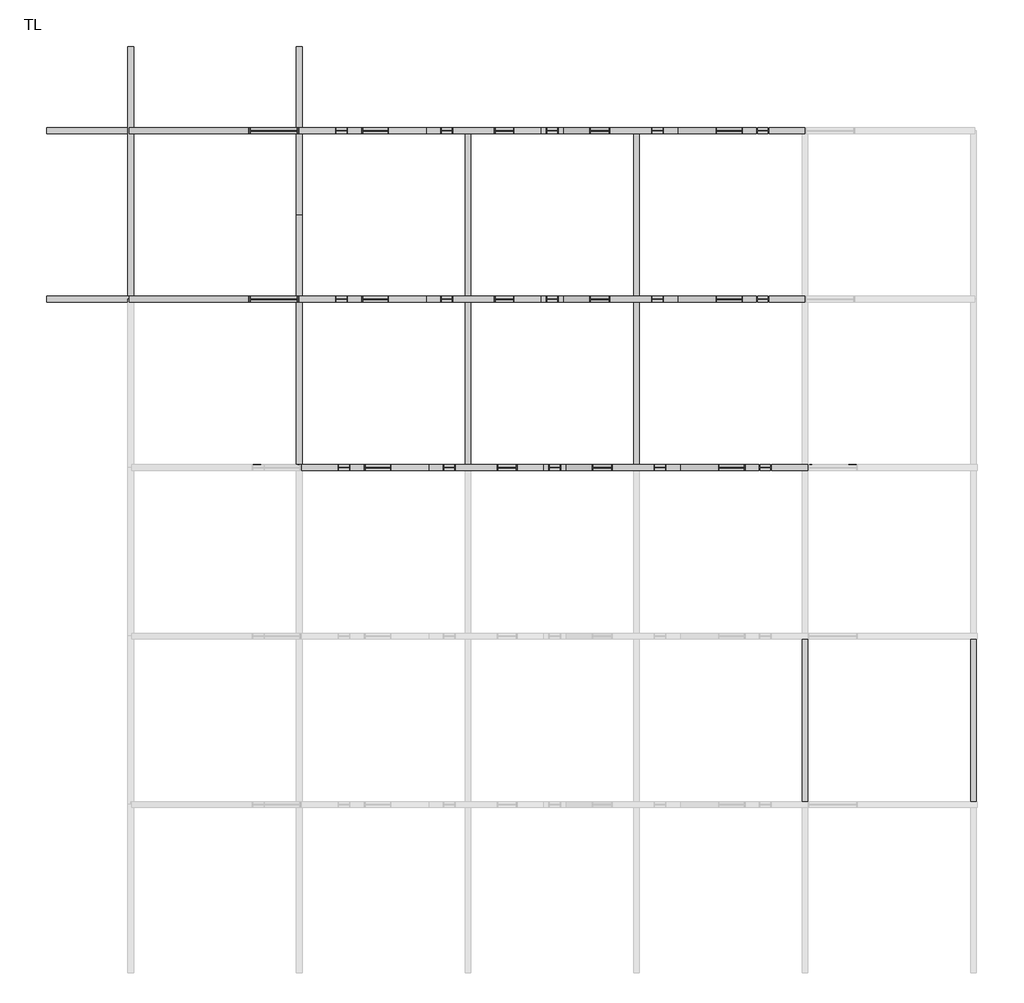
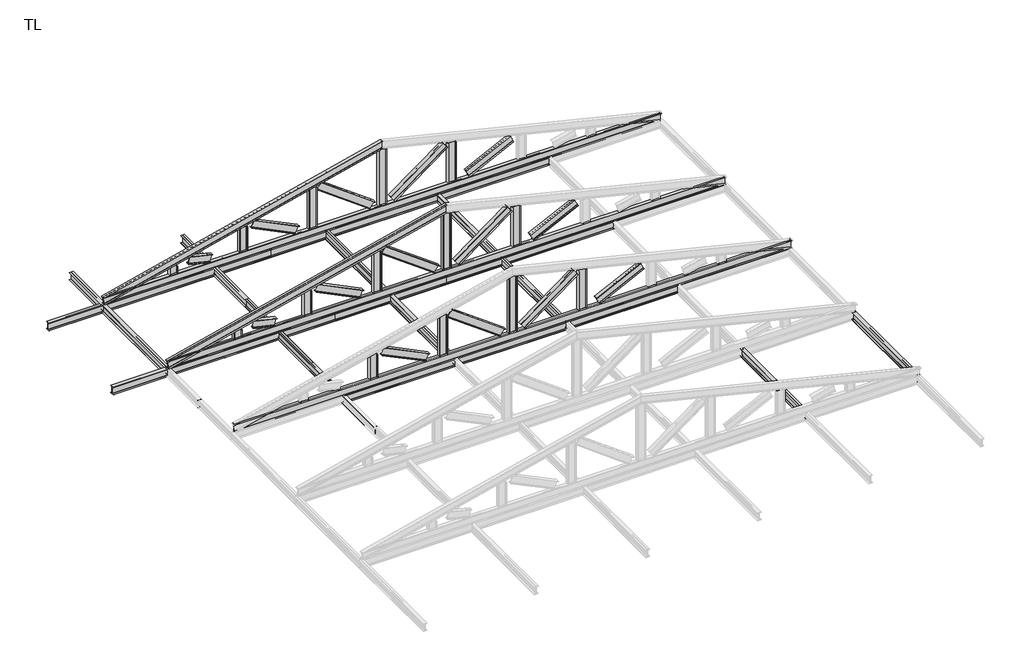
# One storey, part 3 of 4: 53 beams.
"""IFC4 building model written with IfcOpenShell, lengths in millimetres."""

from ifc_helpers import new_model, si_unit, frame, origin, place, context, project, spatial, polyline, circle_curve, ellipse_curve, transform, mapped, element, save
from ifc_brep_helpers import plane_surface, revolved_surface, advanced_brep
from components import w_shapes_w14x30_541e514d, w_shapes_w14x30_920474df, w_shapes_w14x30_f0ef5163, w_shapes_w14x30_e8a2e8cf, w_shapes_w14x30_72b19b1b, w_shapes_w14x30_b44ec7f2, w_shapes_w14x30_809da129, w_shapes_w14x30_b6c746c8, w_shapes_w14x30_333ad3b1, w_shapes_w14x30_a113fbeb, w_shapes_w14x30_23e28ad8, w_shapes_w14x30_8f152a7c

model = new_model("IFC4")

# Units and contexts
model_context = context("Model", 3, world=origin())
ifc_project = project(units=[si_unit("LENGTHUNIT", "METRE", prefix="MILLI")], contexts=[model_context])

# Site, building, storey
site = spatial("IfcSite", under=ifc_project)
building = spatial("IfcBuilding", under=site)
storey = spatial("IfcBuildingStorey", under=building, Name="TL", Elevation=8534.4)

# Beams
placement = place(None, origin())
element("IfcBeam", 1, ObjectType="W Shapes : W14X30", at=placement, inside=storey, context=model_context, shape_type="AdvancedBrep", body=[
    advanced_brep(
    [(-18386.4356148, 14124.3335479, 8538.7295322), (-18384.1189802, 14124.3335479, 8529.2288983), (-18384.1189802, 13953.3915479, 8529.2288983), (-18386.4356148, 13953.3915479, 8538.7295322), (-18386.4356148, 14025.2735479, 8538.7295322), (-18388.8425079, 14035.4335479, 8548.6003207), (-18462.4332635, 14035.4335479, 8850.3996793), (-18464.8401565, 14025.2735479, 8860.2704678), (-18464.8401565, 13953.3915479, 8860.2704678), (-18467.1567911, 13953.3915479, 8869.7711017), (-18467.1567911, 14124.3335479, 8869.7711017), (-18464.8401565, 14124.3335479, 8860.2704678), (-18464.8401565, 14052.4515479, 8860.2704678), (-18462.4332635, 14042.2915479, 8850.3996793), (-18388.8425079, 14042.2915479, 8548.6003207), (-18386.4356148, 14052.4515479, 8538.7295322), (-5925.6378857, 14052.4515479, 11577.1704505), (-5925.6378857, 14124.3335479, 11577.1704505), (-5925.6378857, 14042.2915479, 11587.6281358), (-5925.6378857, 14042.2915479, 11907.3718642), (-5925.6378857, 14052.4515479, 11917.8295495), (-5925.6378857, 14124.3335479, 11917.8295495), (-5925.6378857, 14124.3335479, 11927.8950717), (-5925.6378857, 13953.3915479, 11927.8950717), (-5925.6378857, 13953.3915479, 11917.8295495), (-5925.6378857, 14025.2735479, 11917.8295495), (-5925.6378857, 14035.4335479, 11907.3718642), (-5925.6378857, 14035.4335479, 11587.6281358), (-5925.6378857, 14025.2735479, 11577.1704505), (-5925.6378857, 13953.3915479, 11577.1704505), (-5925.6378857, 13953.3915479, 11567.1049283), (-5925.6378857, 14124.3335479, 11567.1049283)],
    [
        (0, 1),
        (1, 2),
        (2, 3),
        (3, 4),
        (4, 5, circle_curve(frame((-18388.8425079, 14025.2735479, 8548.6003207), z_axis=(0.971534301878756, 0.0, 0.23689892417011604), x_axis=(0.23689892417011604, 0.0, -0.971534301878756)), 10.16)),
        (5, 6),
        (6, 7, circle_curve(frame((-18462.4332635, 14025.2735479, 8850.3996793), z_axis=(0.971534301878756, 0.0, 0.23689892417011604), x_axis=(0.0, 1.0000000000000002, 0.0)), 10.16)),
        (7, 8),
        (8, 9),
        (9, 10),
        (10, 11),
        (11, 12),
        (12, 13, circle_curve(frame((-18462.4332635, 14052.4515479, 8850.3996793), z_axis=(0.971534301878756, 0.0, 0.23689892417011604), x_axis=(-0.23689892417011604, 0.0, 0.971534301878756)), 10.16)),
        (13, 14),
        (14, 15, circle_curve(frame((-18388.8425079, 14052.4515479, 8548.6003207), z_axis=(0.971534301878756, 0.0, 0.23689892417011604), x_axis=(0.0, -1.0000000000000002, 0.0)), 10.16)),
        (15, 0),
        (16, 17),
        (17, 0),
        (15, 16),
        (18, 16, ellipse_curve(frame((-5925.6378857, 14052.4515479, 11587.6281358), z_axis=(1.0, 0.0, 0.0), x_axis=(0.0, 0.0, -1.0)), 10.4576853, 10.16)),
        (14, 18),
        (19, 18),
        (13, 19),
        (20, 19, ellipse_curve(frame((-5925.6378857, 14052.4515479, 11907.3718642), z_axis=(1.0, 0.0, 0.0), x_axis=(0.0, 0.0, -1.0)), 10.4576853, 10.16)),
        (12, 20),
        (21, 20),
        (11, 21),
        (22, 21),
        (10, 22),
        (23, 22),
        (9, 23),
        (24, 23),
        (8, 24),
        (25, 24),
        (7, 25),
        (26, 25, ellipse_curve(frame((-5925.6378857, 14025.2735479, 11907.3718642), z_axis=(1.0, 0.0, 0.0), x_axis=(0.0, 0.0, -1.0)), 10.4576853, 10.16)),
        (6, 26),
        (27, 26),
        (5, 27),
        (28, 27, ellipse_curve(frame((-5925.6378857, 14025.2735479, 11587.6281358), z_axis=(1.0, 0.0, 0.0), x_axis=(0.0, 0.0, -1.0)), 10.4576853, 10.16)),
        (4, 28),
        (29, 28),
        (3, 29),
        (30, 29),
        (2, 30),
        (31, 30),
        (1, 31),
        (17, 31),
    ],
    [
        plane_surface(frame((-18425.6378857, 14038.8625479, 8699.5), z_axis=(-0.971534301878756, 0.0, -0.23689892417011604), x_axis=(-0.23689892417011604, 0.0, 0.971534301878756))),
        plane_surface(frame((-5886.4356148, 14088.3925479, 11586.7295322), z_axis=(-0.23689892417011604, 0.0, 0.971534301878756), x_axis=(0.0, -1.0, 0.0))),
        revolved_surface(polyline([(-18388.8425079, 14042.2915479, 8548.600320699998), (-5923.230992628227, 14042.2915479, 11588.215032583868)]), (-5888.8425079, 14052.4515479, 11596.6003207), (-0.971534301878756, 0.0, -0.23689892417011604)),
        plane_surface(frame((-5925.6378857, 14042.2915479, 11747.5), z_axis=(0.0, 1.0000000000000002, 0.0), x_axis=(-0.23689892417011604, 0.0, 0.971534301878756))),
        revolved_surface(polyline([(-18464.840156569568, 14052.4515479, 8860.270467807088), (-5925.637885708268, 14052.4515479, 11917.82954953391)]), (-5962.4332635, 14052.4515479, 11898.3996793), (-0.971534301878756, 0.0, -0.23689892417011604)),
        plane_surface(frame((-5964.8401565, 14088.3925479, 11908.2704678), z_axis=(0.23689892417011604, 0.0, -0.971534301878756), x_axis=(0.0, 1.0, 0.0))),
        plane_surface(frame((-5965.9984738, 14124.3335479, 11913.0207848), z_axis=(0.0, 1.0000000000000002, 0.0), x_axis=(-0.23689892417011604, 0.0, 0.971534301878756))),
        plane_surface(frame((-5967.1567911, 14038.8625479, 11917.7711017), z_axis=(-0.23689892417011604, 0.0, 0.971534301878756), x_axis=(0.0, -1.0, 0.0))),
        plane_surface(frame((-5965.9984738, 13953.3915479, 11913.0207848), z_axis=(0.0, -1.0000000000000002, 0.0), x_axis=(0.23689892417011604, 0.0, -0.971534301878756))),
        plane_surface(frame((-5964.8401565, 13989.3325479, 11908.2704678), z_axis=(0.23689892417011604, 0.0, -0.971534301878756), x_axis=(0.0, 1.0, 0.0))),
        revolved_surface(polyline([(-18462.4332635, 14035.4335479, 8850.399679299999), (-5923.2309926387, 14035.4335479, 11907.95876102682)]), (-5962.4332635, 14025.2735479, 11898.3996793), (-0.971534301878756, 0.0, -0.23689892417011604)),
        plane_surface(frame((-5925.6378857, 14035.4335479, 11747.5), z_axis=(0.0, -1.0000000000000002, 0.0), x_axis=(0.23689892417011604, 0.0, -0.971534301878756))),
        revolved_surface(polyline([(-18386.435614830432, 14025.2735479, 8538.729532192909), (-5920.824099558658, 14025.2735479, 11578.34424407678)]), (-5888.8425079, 14025.2735479, 11596.6003207), (-0.971534301878756, 0.0, -0.23689892417011604)),
        plane_surface(frame((-5886.4356148, 13989.3325479, 11586.7295322), z_axis=(-0.23689892417011604, 0.0, 0.971534301878756), x_axis=(0.0, -1.0, 0.0))),
        plane_surface(frame((-5885.2772975, 13953.3915479, 11581.9792152), z_axis=(0.0, -1.0000000000000002, 0.0), x_axis=(0.23689892417011604, 0.0, -0.971534301878756))),
        plane_surface(frame((-5884.1189802, 14038.8625479, 11577.2288983), z_axis=(0.23689892417011604, 0.0, -0.971534301878756), x_axis=(0.0, 1.0, 0.0))),
        plane_surface(frame((-5885.2772975, 14124.3335479, 11581.9792152), z_axis=(0.0, 1.0000000000000002, 0.0), x_axis=(-0.23689892417011604, 0.0, 0.971534301878756))),
        plane_surface(frame((-5925.6378857, 14038.8625479, 11927.8950717), z_axis=(1.0, 0.0, 0.0), x_axis=(0.0, -1.0, 0.0))),
    ],
    [
        (0, [[1, 2, 3, 4, 5, 6, 7, 8, 9, 10, 11, 12, 13, 14, 15, 16]]),
        (1, [[17, 18, -16, 19]]),
        (2, [[20, -19, -15, 21]]),
        (3, [[22, -21, -14, 23]]),
        (4, [[24, -23, -13, 25]]),
        (5, [[26, -25, -12, 27]]),
        (6, [[28, -27, -11, 29]]),
        (7, [[30, -29, -10, 31]]),
        (8, [[32, -31, -9, 33]]),
        (9, [[34, -33, -8, 35]]),
        (10, [[36, -35, -7, 37]]),
        (11, [[38, -37, -6, 39]]),
        (12, [[40, -39, -5, 41]]),
        (13, [[42, -41, -4, 43]]),
        (14, [[44, -43, -3, 45]]),
        (15, [[46, -45, -2, 47]]),
        (16, [[48, -47, -1, -18]]),
        (17, [[-17, -20, -22, -24, -26, -28, -30, -32, -34, -36, -38, -40, -42, -44, -46, -48]]),
    ],
),
])
element("IfcBeam", 2, ObjectType="W Shapes : W14X30", at=placement, inside=storey, context=model_context, shape_type="AdvancedBrep", body=[
    advanced_brep(
    [(-18386.4356148, 19124.3335479, 8538.7295322), (-18384.1189802, 19124.3335479, 8529.2288983), (-18384.1189802, 18953.3915479, 8529.2288983), (-18386.4356148, 18953.3915479, 8538.7295322), (-18386.4356148, 19025.2735479, 8538.7295322), (-18388.8425079, 19035.4335479, 8548.6003207), (-18462.4332635, 19035.4335479, 8850.3996793), (-18464.8401565, 19025.2735479, 8860.2704678), (-18464.8401565, 18953.3915479, 8860.2704678), (-18467.1567911, 18953.3915479, 8869.7711017), (-18467.1567911, 19124.3335479, 8869.7711017), (-18464.8401565, 19124.3335479, 8860.2704678), (-18464.8401565, 19052.4515479, 8860.2704678), (-18462.4332635, 19042.2915479, 8850.3996793), (-18388.8425079, 19042.2915479, 8548.6003207), (-18386.4356148, 19052.4515479, 8538.7295322), (-5925.6378857, 19052.4515479, 11577.1704505), (-5925.6378857, 19124.3335479, 11577.1704505), (-5925.6378857, 19042.2915479, 11587.6281358), (-5925.6378857, 19042.2915479, 11907.3718642), (-5925.6378857, 19052.4515479, 11917.8295495), (-5925.6378857, 19124.3335479, 11917.8295495), (-5925.6378857, 19124.3335479, 11927.8950717), (-5925.6378857, 18953.3915479, 11927.8950717), (-5925.6378857, 18953.3915479, 11917.8295495), (-5925.6378857, 19025.2735479, 11917.8295495), (-5925.6378857, 19035.4335479, 11907.3718642), (-5925.6378857, 19035.4335479, 11587.6281358), (-5925.6378857, 19025.2735479, 11577.1704505), (-5925.6378857, 18953.3915479, 11577.1704505), (-5925.6378857, 18953.3915479, 11567.1049283), (-5925.6378857, 19124.3335479, 11567.1049283)],
    [
        (0, 1),
        (1, 2),
        (2, 3),
        (3, 4),
        (4, 5, circle_curve(frame((-18388.8425079, 19025.2735479, 8548.6003207), z_axis=(0.971534301878756, 0.0, 0.23689892417011604), x_axis=(0.23689892417011604, 0.0, -0.971534301878756)), 10.16)),
        (5, 6),
        (6, 7, circle_curve(frame((-18462.4332635, 19025.2735479, 8850.3996793), z_axis=(0.971534301878756, 0.0, 0.23689892417011604), x_axis=(0.0, 1.0000000000000002, 0.0)), 10.16)),
        (7, 8),
        (8, 9),
        (9, 10),
        (10, 11),
        (11, 12),
        (12, 13, circle_curve(frame((-18462.4332635, 19052.4515479, 8850.3996793), z_axis=(0.971534301878756, 0.0, 0.23689892417011604), x_axis=(-0.23689892417011604, 0.0, 0.971534301878756)), 10.16)),
        (13, 14),
        (14, 15, circle_curve(frame((-18388.8425079, 19052.4515479, 8548.6003207), z_axis=(0.971534301878756, 0.0, 0.23689892417011604), x_axis=(0.0, -1.0000000000000002, 0.0)), 10.16)),
        (15, 0),
        (16, 17),
        (17, 0),
        (15, 16),
        (18, 16, ellipse_curve(frame((-5925.6378857, 19052.4515479, 11587.6281358), z_axis=(1.0, 0.0, 0.0), x_axis=(0.0, 0.0, -1.0)), 10.4576853, 10.16)),
        (14, 18),
        (19, 18),
        (13, 19),
        (20, 19, ellipse_curve(frame((-5925.6378857, 19052.4515479, 11907.3718642), z_axis=(1.0, 0.0, 0.0), x_axis=(0.0, 0.0, -1.0)), 10.4576853, 10.16)),
        (12, 20),
        (21, 20),
        (11, 21),
        (22, 21),
        (10, 22),
        (23, 22),
        (9, 23),
        (24, 23),
        (8, 24),
        (25, 24),
        (7, 25),
        (26, 25, ellipse_curve(frame((-5925.6378857, 19025.2735479, 11907.3718642), z_axis=(1.0, 0.0, 0.0), x_axis=(0.0, 0.0, -1.0)), 10.4576853, 10.16)),
        (6, 26),
        (27, 26),
        (5, 27),
        (28, 27, ellipse_curve(frame((-5925.6378857, 19025.2735479, 11587.6281358), z_axis=(1.0, 0.0, 0.0), x_axis=(0.0, 0.0, -1.0)), 10.4576853, 10.16)),
        (4, 28),
        (29, 28),
        (3, 29),
        (30, 29),
        (2, 30),
        (31, 30),
        (1, 31),
        (17, 31),
    ],
    [
        plane_surface(frame((-18425.6378857, 19038.8625479, 8699.5), z_axis=(-0.971534301878756, 0.0, -0.23689892417011604), x_axis=(-0.23689892417011604, 0.0, 0.971534301878756))),
        plane_surface(frame((-5886.4356148, 19088.3925479, 11586.7295322), z_axis=(-0.23689892417011604, 0.0, 0.971534301878756), x_axis=(0.0, -1.0, 0.0))),
        revolved_surface(polyline([(-18388.8425079, 19042.2915479, 8548.600320699998), (-5923.230992628227, 19042.2915479, 11588.215032583868)]), (-5888.8425079, 19052.4515479, 11596.6003207), (-0.971534301878756, 0.0, -0.23689892417011604)),
        plane_surface(frame((-5925.6378857, 19042.2915479, 11747.5), z_axis=(0.0, 1.0000000000000002, 0.0), x_axis=(-0.23689892417011604, 0.0, 0.971534301878756))),
        revolved_surface(polyline([(-18464.840156569568, 19052.4515479, 8860.270467807088), (-5925.637885708268, 19052.4515479, 11917.82954953391)]), (-5962.4332635, 19052.4515479, 11898.3996793), (-0.971534301878756, 0.0, -0.23689892417011604)),
        plane_surface(frame((-5964.8401565, 19088.3925479, 11908.2704678), z_axis=(0.23689892417011604, 0.0, -0.971534301878756), x_axis=(0.0, 1.0, 0.0))),
        plane_surface(frame((-5965.9984738, 19124.3335479, 11913.0207848), z_axis=(0.0, 1.0000000000000002, 0.0), x_axis=(-0.23689892417011604, 0.0, 0.971534301878756))),
        plane_surface(frame((-5967.1567911, 19038.8625479, 11917.7711017), z_axis=(-0.23689892417011604, 0.0, 0.971534301878756), x_axis=(0.0, -1.0, 0.0))),
        plane_surface(frame((-5965.9984738, 18953.3915479, 11913.0207848), z_axis=(0.0, -1.0000000000000002, 0.0), x_axis=(0.23689892417011604, 0.0, -0.971534301878756))),
        plane_surface(frame((-5964.8401565, 18989.3325479, 11908.2704678), z_axis=(0.23689892417011604, 0.0, -0.971534301878756), x_axis=(0.0, 1.0, 0.0))),
        revolved_surface(polyline([(-18462.4332635, 19035.4335479, 8850.399679299999), (-5923.2309926387, 19035.4335479, 11907.95876102682)]), (-5962.4332635, 19025.2735479, 11898.3996793), (-0.971534301878756, 0.0, -0.23689892417011604)),
        plane_surface(frame((-5925.6378857, 19035.4335479, 11747.5), z_axis=(0.0, -1.0000000000000002, 0.0), x_axis=(0.23689892417011604, 0.0, -0.971534301878756))),
        revolved_surface(polyline([(-18386.435614830432, 19025.2735479, 8538.729532192909), (-5920.824099558658, 19025.2735479, 11578.34424407678)]), (-5888.8425079, 19025.2735479, 11596.6003207), (-0.971534301878756, 0.0, -0.23689892417011604)),
        plane_surface(frame((-5886.4356148, 18989.3325479, 11586.7295322), z_axis=(-0.23689892417011604, 0.0, 0.971534301878756), x_axis=(0.0, -1.0, 0.0))),
        plane_surface(frame((-5885.2772975, 18953.3915479, 11581.9792152), z_axis=(0.0, -1.0000000000000002, 0.0), x_axis=(0.23689892417011604, 0.0, -0.971534301878756))),
        plane_surface(frame((-5884.1189802, 19038.8625479, 11577.2288983), z_axis=(0.23689892417011604, 0.0, -0.971534301878756), x_axis=(0.0, 1.0, 0.0))),
        plane_surface(frame((-5885.2772975, 19124.3335479, 11581.9792152), z_axis=(0.0, 1.0000000000000002, 0.0), x_axis=(-0.23689892417011604, 0.0, 0.971534301878756))),
        plane_surface(frame((-5925.6378857, 19038.8625479, 11927.8950717), z_axis=(1.0, 0.0, 0.0), x_axis=(0.0, -1.0, 0.0))),
    ],
    [
        (0, [[1, 2, 3, 4, 5, 6, 7, 8, 9, 10, 11, 12, 13, 14, 15, 16]]),
        (1, [[17, 18, -16, 19]]),
        (2, [[20, -19, -15, 21]]),
        (3, [[22, -21, -14, 23]]),
        (4, [[24, -23, -13, 25]]),
        (5, [[26, -25, -12, 27]]),
        (6, [[28, -27, -11, 29]]),
        (7, [[30, -29, -10, 31]]),
        (8, [[32, -31, -9, 33]]),
        (9, [[34, -33, -8, 35]]),
        (10, [[36, -35, -7, 37]]),
        (11, [[38, -37, -6, 39]]),
        (12, [[40, -39, -5, 41]]),
        (13, [[42, -41, -4, 43]]),
        (14, [[44, -43, -3, 45]]),
        (15, [[46, -45, -2, 47]]),
        (16, [[48, -47, -1, -18]]),
        (17, [[-17, -20, -22, -24, -26, -28, -30, -32, -34, -36, -38, -40, -42, -44, -46, -48]]),
    ],
),
])
w_shapes_w14x30_shape = w_shapes_w14x30_541e514d(model_context)
element("IfcBeam", 3, ObjectType="W Shapes : W14X30", at=placement, inside=storey, context=model_context, shape_type="MappedRepresentation", body=[
    mapped(w_shapes_w14x30_shape, transform((-15925.6378857, 14038.8625479, 8359.14), x_axis=(1.0, 0.0, 0.0), y_axis=(0.0, 1.0, 0.0), z_axis=(0.0, 0.0, 1.0))),
])
element("IfcBeam", 4, ObjectType="W Shapes : W14X30", at=placement, inside=storey, context=model_context, shape_type="MappedRepresentation", body=[
    mapped(w_shapes_w14x30_shape, transform((-15925.6378857, 19038.8625479, 8359.14), x_axis=(1.0, 0.0, 0.0), y_axis=(0.0, 1.0, 0.0), z_axis=(0.0, 0.0, 1.0))),
])
element("IfcBeam", 5, ObjectType="W Shapes : W14X30", at=placement, inside=storey, context=model_context, shape_type="MappedRepresentation", body=[
    mapped(w_shapes_w14x30_shape, transform((-13425.6378857, 11538.8625479, 8359.14), x_axis=(0.0, 1.0, 0.0), y_axis=(-1.0, 0.0, 0.0), z_axis=(0.0, 0.0, 1.0))),
])
element("IfcBeam", 6, ObjectType="W Shapes : W14X30", at=placement, inside=storey, context=model_context, shape_type="MappedRepresentation", body=[
    mapped(w_shapes_w14x30_shape, transform((-13425.6378857, 16538.8625479, 8359.14), x_axis=(0.0, 1.0, 0.0), y_axis=(-1.0, 0.0, 0.0), z_axis=(0.0, 0.0, 1.0))),
])
element("IfcBeam", 7, ObjectType="W Shapes : W14X30", at=placement, inside=storey, context=model_context, shape_type="MappedRepresentation", body=[
    mapped(w_shapes_w14x30_shape, transform((-18425.6378857, 16538.8625479, 8359.14), x_axis=(0.0, 1.0, 0.0), y_axis=(-1.0, 0.0, 0.0), z_axis=(0.0, 0.0, 1.0))),
])
element("IfcBeam", 8, ObjectType="W Shapes : W14X30", at=placement, inside=storey, context=model_context, shape_type="MappedRepresentation", body=[
    mapped(w_shapes_w14x30_shape, transform((-10925.6378857, 14038.8625479, 8359.14), x_axis=(1.0, 0.0, 0.0), y_axis=(0.0, 1.0, 0.0), z_axis=(0.0, 0.0, 1.0))),
])
w_shapes_w14x30_2_shape = w_shapes_w14x30_920474df(model_context)
element("IfcBeam", 9, ObjectType="W Shapes : W14X30", at=placement, inside=storey, context=model_context, shape_type="MappedRepresentation", body=[
    mapped(w_shapes_w14x30_2_shape, transform((-10925.6378857, 9038.8625479, 8359.14), x_axis=(1.0, 0.0, 0.0), y_axis=(0.0, 1.0, 0.0), z_axis=(0.0, 0.0, 1.0))),
])
element("IfcBeam", 10, ObjectType="W Shapes : W14X30", at=placement, inside=storey, context=model_context, shape_type="MappedRepresentation", body=[
    mapped(w_shapes_w14x30_2_shape, transform((-5925.6378857, 9038.8625479, 8359.14), x_axis=(1.0, 0.0, 0.0), y_axis=(0.0, 1.0, 0.0), z_axis=(0.0, 0.0, 1.0))),
])
element("IfcBeam", 11, ObjectType="W Shapes : W14X30", at=placement, inside=storey, context=model_context, shape_type="MappedRepresentation", body=[
    mapped(w_shapes_w14x30_2_shape, transform((-925.6378857, 9038.8625479, 8359.14), x_axis=(1.0, 0.0, 0.0), y_axis=(0.0, 1.0, 0.0), z_axis=(0.0, 0.0, 1.0))),
])
element("IfcBeam", 12, ObjectType="W Shapes : W14X30", at=placement, inside=storey, context=model_context, shape_type="MappedRepresentation", body=[
    mapped(w_shapes_w14x30_2_shape, transform((-5925.6378857, 14038.8625479, 8359.14), x_axis=(1.0, 0.0, 0.0), y_axis=(0.0, 1.0, 0.0), z_axis=(0.0, 0.0, 1.0))),
])
element("IfcBeam", 13, ObjectType="W Shapes : W14X30", at=placement, inside=storey, context=model_context, shape_type="MappedRepresentation", body=[
    mapped(w_shapes_w14x30_2_shape, transform((-925.6378857, 14038.8625479, 8359.14), x_axis=(1.0, 0.0, 0.0), y_axis=(0.0, 1.0, 0.0), z_axis=(0.0, 0.0, 1.0))),
])
element("IfcBeam", 14, ObjectType="W Shapes : W14X30", at=placement, inside=storey, context=model_context, shape_type="MappedRepresentation", body=[
    mapped(w_shapes_w14x30_2_shape, transform((-10925.6378857, 19038.8625479, 8359.14), x_axis=(1.0, 0.0, 0.0), y_axis=(0.0, 1.0, 0.0), z_axis=(0.0, 0.0, 1.0))),
])
element("IfcBeam", 15, ObjectType="W Shapes : W14X30", at=placement, inside=storey, context=model_context, shape_type="MappedRepresentation", body=[
    mapped(w_shapes_w14x30_2_shape, transform((-5925.6378857, 19038.8625479, 8359.14), x_axis=(1.0, 0.0, 0.0), y_axis=(0.0, 1.0, 0.0), z_axis=(0.0, 0.0, 1.0))),
])
element("IfcBeam", 16, ObjectType="W Shapes : W14X30", at=placement, inside=storey, context=model_context, shape_type="MappedRepresentation", body=[
    mapped(w_shapes_w14x30_2_shape, transform((-925.6378857, 19038.8625479, 8359.14), x_axis=(1.0, 0.0, 0.0), y_axis=(0.0, 1.0, 0.0), z_axis=(0.0, 0.0, 1.0))),
])
element("IfcBeam", 17, ObjectType="W Shapes : W14X30", at=placement, inside=storey, context=model_context, shape_type="MappedRepresentation", body=[
    mapped(w_shapes_w14x30_2_shape, transform((6574.3621143, 1538.8625479, 8359.14), x_axis=(0.0, 1.0, 0.0), y_axis=(-1.0, 0.0, 0.0), z_axis=(0.0, 0.0, 1.0))),
])
element("IfcBeam", 18, ObjectType="W Shapes : W14X30", at=placement, inside=storey, context=model_context, shape_type="MappedRepresentation", body=[
    mapped(w_shapes_w14x30_2_shape, transform((1574.3621143, 1538.8625479, 8359.14), x_axis=(0.0, 1.0, 0.0), y_axis=(-1.0, 0.0, 0.0), z_axis=(0.0, 0.0, 1.0))),
])
element("IfcBeam", 19, ObjectType="W Shapes : W14X30", at=placement, inside=storey, context=model_context, shape_type="MappedRepresentation", body=[
    mapped(w_shapes_w14x30_2_shape, transform((-3425.6378857, 11538.8625479, 8359.14), x_axis=(0.0, 1.0, 0.0), y_axis=(-1.0, 0.0, 0.0), z_axis=(0.0, 0.0, 1.0))),
])
element("IfcBeam", 20, ObjectType="W Shapes : W14X30", at=placement, inside=storey, context=model_context, shape_type="MappedRepresentation", body=[
    mapped(w_shapes_w14x30_2_shape, transform((-3425.6378857, 16538.8625479, 8359.14), x_axis=(0.0, 1.0, 0.0), y_axis=(-1.0, 0.0, 0.0), z_axis=(0.0, 0.0, 1.0))),
])
element("IfcBeam", 21, ObjectType="W Shapes : W14X30", at=placement, inside=storey, context=model_context, shape_type="MappedRepresentation", body=[
    mapped(w_shapes_w14x30_2_shape, transform((-8425.6378857, 11538.8625479, 8359.14), x_axis=(0.0, 1.0, 0.0), y_axis=(-1.0, 0.0, 0.0), z_axis=(0.0, 0.0, 1.0))),
])
element("IfcBeam", 22, ObjectType="W Shapes : W14X30", at=placement, inside=storey, context=model_context, shape_type="MappedRepresentation", body=[
    mapped(w_shapes_w14x30_2_shape, transform((-8425.6378857, 16538.8625479, 8359.14), x_axis=(0.0, 1.0, 0.0), y_axis=(-1.0, 0.0, 0.0), z_axis=(0.0, 0.0, 1.0))),
])
w_shapes_w14x30_3_shape = w_shapes_w14x30_f0ef5163(model_context)
element("IfcBeam", 23, ObjectType="W Shapes : W14X30", at=placement, inside=storey, context=model_context, shape_type="MappedRepresentation", body=[
    mapped(w_shapes_w14x30_3_shape, transform((-5925.6378857, 14038.8625479, 8699.5), x_axis=(1.0, 0.0, 0.0), y_axis=(0.0, 1.0, 0.0), z_axis=(0.0, 0.0, 1.0))),
])
element("IfcBeam", 24, ObjectType="W Shapes : W14X30", at=placement, inside=storey, context=model_context, shape_type="MappedRepresentation", body=[
    mapped(w_shapes_w14x30_3_shape, transform((-5849.4378857, 9038.8625479, 8699.5), x_axis=(1.0, 0.0, 0.0), y_axis=(0.0, 1.0, 0.0), z_axis=(0.0, 0.0, 1.0))),
])
element("IfcBeam", 25, ObjectType="W Shapes : W14X30", at=placement, inside=storey, context=model_context, shape_type="MappedRepresentation", body=[
    mapped(w_shapes_w14x30_3_shape, transform((-5925.6378857, 19038.8625479, 8699.5), x_axis=(1.0, 0.0, 0.0), y_axis=(0.0, 1.0, 0.0), z_axis=(0.0, 0.0, 1.0))),
])
w_shapes_w14x30_4_shape = w_shapes_w14x30_e8a2e8cf(model_context)
element("IfcBeam", 26, ObjectType="W Shapes : W14X30", at=placement, inside=storey, context=model_context, shape_type="MappedRepresentation", body=[
    mapped(w_shapes_w14x30_4_shape, transform((-5925.6378857, 14038.8625479, 10223.5), x_axis=(0.0, 0.0, 1.0), y_axis=(0.0, -1.0, 0.0), z_axis=(1.0, 0.0, 0.0))),
])
element("IfcBeam", 27, ObjectType="W Shapes : W14X30", at=placement, inside=storey, context=model_context, shape_type="MappedRepresentation", body=[
    mapped(w_shapes_w14x30_4_shape, transform((-5849.4378857, 9038.8625479, 10223.5), x_axis=(0.0, 0.0, 1.0), y_axis=(0.0, -1.0, 0.0), z_axis=(1.0, 0.0, 0.0))),
])
element("IfcBeam", 28, ObjectType="W Shapes : W14X30", at=placement, inside=storey, context=model_context, shape_type="MappedRepresentation", body=[
    mapped(w_shapes_w14x30_4_shape, transform((-5925.6378857, 19038.8625479, 10223.5), x_axis=(0.0, 0.0, 1.0), y_axis=(0.0, -1.0, 0.0), z_axis=(1.0, 0.0, 0.0))),
])
w_shapes_w14x30_5_shape = w_shapes_w14x30_72b19b1b(model_context)
element("IfcBeam", 29, ObjectType="W Shapes : W14X30", at=placement, inside=storey, context=model_context, shape_type="MappedRepresentation", body=[
    mapped(w_shapes_w14x30_5_shape, transform((-9050.6378857, 14038.8625479, 9842.5), x_axis=(0.0, 0.0, 1.0), y_axis=(0.0, -1.0, 0.0), z_axis=(1.0, 0.0, 0.0))),
])
element("IfcBeam", 30, ObjectType="W Shapes : W14X30", at=placement, inside=storey, context=model_context, shape_type="MappedRepresentation", body=[
    mapped(w_shapes_w14x30_5_shape, transform((-2800.6378857, 14038.8625479, 9842.5), x_axis=(0.0, 0.0, 1.0), y_axis=(0.0, -1.0, 0.0), z_axis=(1.0, 0.0, 0.0))),
])
element("IfcBeam", 31, ObjectType="W Shapes : W14X30", at=placement, inside=storey, context=model_context, shape_type="MappedRepresentation", body=[
    mapped(w_shapes_w14x30_5_shape, transform((-8974.4378857, 9038.8625479, 9842.5), x_axis=(0.0, 0.0, 1.0), y_axis=(0.0, -1.0, 0.0), z_axis=(1.0, 0.0, 0.0))),
])
element("IfcBeam", 32, ObjectType="W Shapes : W14X30", at=placement, inside=storey, context=model_context, shape_type="MappedRepresentation", body=[
    mapped(w_shapes_w14x30_5_shape, transform((-2724.4378857, 9038.8625479, 9842.5), x_axis=(0.0, 0.0, 1.0), y_axis=(0.0, -1.0, 0.0), z_axis=(1.0, 0.0, 0.0))),
])
element("IfcBeam", 33, ObjectType="W Shapes : W14X30", at=placement, inside=storey, context=model_context, shape_type="MappedRepresentation", body=[
    mapped(w_shapes_w14x30_5_shape, transform((-9050.6378857, 19038.8625479, 9842.5), x_axis=(0.0, 0.0, 1.0), y_axis=(0.0, -1.0, 0.0), z_axis=(1.0, 0.0, 0.0))),
])
element("IfcBeam", 34, ObjectType="W Shapes : W14X30", at=placement, inside=storey, context=model_context, shape_type="MappedRepresentation", body=[
    mapped(w_shapes_w14x30_5_shape, transform((-2800.6378857, 19038.8625479, 9842.5), x_axis=(0.0, 0.0, 1.0), y_axis=(0.0, -1.0, 0.0), z_axis=(1.0, 0.0, 0.0))),
])
w_shapes_w14x30_6_shape = w_shapes_w14x30_b44ec7f2(model_context)
element("IfcBeam", 35, ObjectType="W Shapes : W14X30", at=placement, inside=storey, context=model_context, shape_type="MappedRepresentation", body=[
    mapped(w_shapes_w14x30_6_shape, transform((-12175.6378857, 14038.8625479, 9461.5), x_axis=(0.0, 0.0, 1.0), y_axis=(0.0, -1.0, 0.0), z_axis=(1.0, 0.0, 0.0))),
])
element("IfcBeam", 36, ObjectType="W Shapes : W14X30", at=placement, inside=storey, context=model_context, shape_type="MappedRepresentation", body=[
    mapped(w_shapes_w14x30_6_shape, transform((-12099.4378857, 9038.8625479, 9461.5), x_axis=(0.0, 0.0, 1.0), y_axis=(0.0, -1.0, 0.0), z_axis=(1.0, 0.0, 0.0))),
])
element("IfcBeam", 37, ObjectType="W Shapes : W14X30", at=placement, inside=storey, context=model_context, shape_type="MappedRepresentation", body=[
    mapped(w_shapes_w14x30_6_shape, transform((-12175.6378857, 19038.8625479, 9461.5), x_axis=(0.0, 0.0, 1.0), y_axis=(0.0, -1.0, 0.0), z_axis=(1.0, 0.0, 0.0))),
])
w_shapes_w14x30_7_shape = w_shapes_w14x30_809da129(model_context)
element("IfcBeam", 38, ObjectType="W Shapes : W14X30", at=placement, inside=storey, context=model_context, shape_type="MappedRepresentation", body=[
    mapped(w_shapes_w14x30_7_shape, transform((-15300.6378857, 14038.8625479, 9080.5), x_axis=(0.0, 0.0, 1.0), y_axis=(0.0, -1.0, 0.0), z_axis=(1.0, 0.0, 0.0))),
])
element("IfcBeam", 39, ObjectType="W Shapes : W14X30", at=placement, inside=storey, context=model_context, shape_type="MappedRepresentation", body=[
    mapped(w_shapes_w14x30_7_shape, transform((-15300.6378857, 19038.8625479, 9080.5), x_axis=(0.0, 0.0, 1.0), y_axis=(0.0, -1.0, 0.0), z_axis=(1.0, 0.0, 0.0))),
])
w_shapes_w14x30_8_shape = w_shapes_w14x30_b6c746c8(model_context)
element("IfcBeam", 40, ObjectType="W Shapes : W14X30", at=placement, inside=storey, context=model_context, shape_type="MappedRepresentation", body=[
    mapped(w_shapes_w14x30_8_shape, transform((-7488.1378857, 14038.8625479, 9842.5), x_axis=(0.8071023678442881, 0.0, -0.5904115241254555), y_axis=(0.0, -1.0, 0.0), z_axis=(-0.5904115241254555, 0.0, -0.8071023678442881))),
])
element("IfcBeam", 41, ObjectType="W Shapes : W14X30", at=placement, inside=storey, context=model_context, shape_type="MappedRepresentation", body=[
    mapped(w_shapes_w14x30_8_shape, transform((-7411.9378857, 9038.8625479, 9842.5), x_axis=(0.8071023678442881, 0.0, -0.5904115241254555), y_axis=(0.0, -1.0, 0.0), z_axis=(-0.5904115241254555, 0.0, -0.8071023678442881))),
])
element("IfcBeam", 42, ObjectType="W Shapes : W14X30", at=placement, inside=storey, context=model_context, shape_type="MappedRepresentation", body=[
    mapped(w_shapes_w14x30_8_shape, transform((-7488.1378857, 19038.8625479, 9842.5), x_axis=(0.8071023678442881, 0.0, -0.5904115241254555), y_axis=(0.0, -1.0, 0.0), z_axis=(-0.5904115241254555, 0.0, -0.8071023678442881))),
])
w_shapes_w14x30_9_shape = w_shapes_w14x30_333ad3b1(model_context)
element("IfcBeam", 43, ObjectType="W Shapes : W14X30", at=placement, inside=storey, context=model_context, shape_type="MappedRepresentation", body=[
    mapped(w_shapes_w14x30_9_shape, transform((-10613.1378857, 14038.8625479, 9461.5), x_axis=(0.8988126690463005, 0.0, -0.4383329624405008), y_axis=(0.0, -1.0, 0.0), z_axis=(-0.4383329624405008, 0.0, -0.8988126690463005))),
])
element("IfcBeam", 44, ObjectType="W Shapes : W14X30", at=placement, inside=storey, context=model_context, shape_type="MappedRepresentation", body=[
    mapped(w_shapes_w14x30_9_shape, transform((-10536.9378857, 9038.8625479, 9461.5), x_axis=(0.8988126690463005, 0.0, -0.4383329624405008), y_axis=(0.0, -1.0, 0.0), z_axis=(-0.4383329624405008, 0.0, -0.8988126690463005))),
])
element("IfcBeam", 45, ObjectType="W Shapes : W14X30", at=placement, inside=storey, context=model_context, shape_type="MappedRepresentation", body=[
    mapped(w_shapes_w14x30_9_shape, transform((-10613.1378857, 19038.8625479, 9461.5), x_axis=(0.8988126690463005, 0.0, -0.4383329624405008), y_axis=(0.0, -1.0, 0.0), z_axis=(-0.4383329624405008, 0.0, -0.8988126690463005))),
])
w_shapes_w14x30_10_shape = w_shapes_w14x30_a113fbeb(model_context)
element("IfcBeam", 46, ObjectType="W Shapes : W14X30", at=placement, inside=storey, context=model_context, shape_type="MappedRepresentation", body=[
    mapped(w_shapes_w14x30_10_shape, transform((-4363.1378857, 14038.8625479, 9842.5), x_axis=(0.8071023678442877, 0.0, 0.590411524125456), y_axis=(0.0, -1.0, 0.0), z_axis=(0.590411524125456, 0.0, -0.8071023678442877))),
])
element("IfcBeam", 47, ObjectType="W Shapes : W14X30", at=placement, inside=storey, context=model_context, shape_type="MappedRepresentation", body=[
    mapped(w_shapes_w14x30_10_shape, transform((-4286.9378857, 9038.8625479, 9842.5), x_axis=(0.8071023678442877, 0.0, 0.590411524125456), y_axis=(0.0, -1.0, 0.0), z_axis=(0.590411524125456, 0.0, -0.8071023678442877))),
])
element("IfcBeam", 48, ObjectType="W Shapes : W14X30", at=placement, inside=storey, context=model_context, shape_type="MappedRepresentation", body=[
    mapped(w_shapes_w14x30_10_shape, transform((-4363.1378857, 19038.8625479, 9842.5), x_axis=(0.8071023678442877, 0.0, 0.590411524125456), y_axis=(0.0, -1.0, 0.0), z_axis=(0.590411524125456, 0.0, -0.8071023678442877))),
])
w_shapes_w14x30_11_shape = w_shapes_w14x30_23e28ad8(model_context)
element("IfcBeam", 49, ObjectType="W Shapes : W14X30", at=placement, inside=storey, context=model_context, shape_type="MappedRepresentation", body=[
    mapped(w_shapes_w14x30_11_shape, transform((-1238.1378857, 14038.8625479, 9461.5), x_axis=(0.8988126690463014, 0.0, 0.4383329624404991), y_axis=(0.0, -1.0, 0.0), z_axis=(0.4383329624404991, 0.0, -0.8988126690463014))),
])
element("IfcBeam", 50, ObjectType="W Shapes : W14X30", at=placement, inside=storey, context=model_context, shape_type="MappedRepresentation", body=[
    mapped(w_shapes_w14x30_11_shape, transform((-1161.9378857, 9038.8625479, 9461.5), x_axis=(0.8988126690463014, 0.0, 0.4383329624404991), y_axis=(0.0, -1.0, 0.0), z_axis=(0.4383329624404991, 0.0, -0.8988126690463014))),
])
element("IfcBeam", 51, ObjectType="W Shapes : W14X30", at=placement, inside=storey, context=model_context, shape_type="MappedRepresentation", body=[
    mapped(w_shapes_w14x30_11_shape, transform((-1238.1378857, 19038.8625479, 9461.5), x_axis=(0.8988126690463014, 0.0, 0.4383329624404991), y_axis=(0.0, -1.0, 0.0), z_axis=(0.4383329624404991, 0.0, -0.8988126690463014))),
])
w_shapes_w14x30_12_shape = w_shapes_w14x30_8f152a7c(model_context)
element("IfcBeam", 52, ObjectType="W Shapes : W14X30", at=placement, inside=storey, context=model_context, shape_type="MappedRepresentation", body=[
    mapped(w_shapes_w14x30_12_shape, transform((-13738.1378857, 14038.8625479, 9080.5), x_axis=(0.9715343018787559, 0.0, -0.23689892417011585), y_axis=(0.0, -1.0, 0.0), z_axis=(-0.23689892417011585, 0.0, -0.9715343018787559))),
])
element("IfcBeam", 53, ObjectType="W Shapes : W14X30", at=placement, inside=storey, context=model_context, shape_type="MappedRepresentation", body=[
    mapped(w_shapes_w14x30_12_shape, transform((-13738.1378857, 19038.8625479, 9080.5), x_axis=(0.9715343018787559, 0.0, -0.23689892417011585), y_axis=(0.0, -1.0, 0.0), z_axis=(-0.23689892417011585, 0.0, -0.9715343018787559))),
])

save(model, "model.ifc")

# Revit data of these elements
# Type "W Shapes : W14X30"
#   Section Name Key = "W14X30"
#   Width = 6.730"
#   Web Thickness = 0.270"
#   Web Fillet = 0.400"
#   Warping Constant = 887.00 in⁶
#   Torsional Moment of Inertia = 0.38 in⁴
#   Section Area = 8.85 in²
#   Plastic Modulus weak axis = 8.99 in³
#   Plastic Modulus strong axis = 47.30 in³
#   Perimeter = 4.441 ft²/ft
#   Nominal Weight = 30.00 lbf/ft
#   Moment of Inertia weak axis = 19.60 in⁴
#   Moment of Inertia strong axis = 291.00 in⁴
#   Height = 13.800"
#   Flange Thickness = 0.385"
#   Elastic Modulus weak axis = 5.82 in³
#   Elastic Modulus strong axis = 42.00 in³
#   Clear Web Height = 0' - 11 5/8"
#   Centroid Vertical = 6.900"
#   Centroid Horizontal = 3.365"
#   Bolt Spacing = 0' - 3 1/2"
#   Length [instance default] = 1524 mm
#   Structural Material [instance default] = Steel ASTM A992
#   Principal Axes Angle = 0
# Elements 1, 2 (IfcBeam, "W Shapes : W14X30")
#   Length = 12866.247 mm
#   Structural Material = Steel ASTM A992
#   Phase Created = New Construction
#   Materials on its faces: "Steel ASTM A992"
# Elements 3, 4, 5, 6, 7, 8, 9, 10, 11, 12, 13, 14, 15, 16, 17, 18, 19, 20, 21, 22 (IfcBeam, "W Shapes : W14X30")
#   Length = 5000 mm
#   Structural Material = Steel ASTM A992
#   Phase Created = New Construction
#   Materials on its faces: "Steel ASTM A992"
# Elements 23, 24, 25 (IfcBeam, "W Shapes : W14X30")
#   Length = 25000 mm
#   Structural Material = Steel ASTM A992
#   Phase Created = New Construction
#   Materials on its faces: "Steel ASTM A992"
# Elements 26, 27, 28 (IfcBeam, "W Shapes : W14X30")
#   Length = 3048 mm
#   Structural Material = Steel ASTM A992
#   Phase Created = New Construction
#   Materials on its faces: "Steel ASTM A992"
# Elements 29, 30, 31, 32, 33, 34 (IfcBeam, "W Shapes : W14X30")
#   Length = 2286 mm
#   Structural Material = Steel ASTM A992
#   Phase Created = New Construction
#   Materials on its faces: "Steel ASTM A992"
# Elements 35, 36, 37 (IfcBeam, "W Shapes : W14X30")
#   Length = 1524 mm
#   Structural Material = Steel ASTM A992
#   Phase Created = New Construction
#   Materials on its faces: "Steel ASTM A992"
# Elements 38, 39 (IfcBeam, "W Shapes : W14X30")
#   Length = 762 mm
#   Structural Material = Steel ASTM A992
#   Phase Created = New Construction
#   Materials on its faces: "Steel ASTM A992"
# Elements 40, 41, 42, 46, 47, 48 (IfcBeam, "W Shapes : W14X30")
#   Length = 3871.876 mm
#   Structural Material = Steel ASTM A992
#   Phase Created = New Construction
#   Materials on its faces: "Steel ASTM A992"
# Elements 43, 44, 45, 49, 50, 51 (IfcBeam, "W Shapes : W14X30")
#   Length = 3476.809 mm
#   Structural Material = Steel ASTM A992
#   Phase Created = New Construction
#   Materials on its faces: "Steel ASTM A992"
# Elements 52, 53 (IfcBeam, "W Shapes : W14X30")
#   Length = 3216.562 mm
#   Structural Material = Steel ASTM A992
#   Phase Created = New Construction
#   Materials on its faces: "Steel ASTM A992"
# Materials
#   "Steel ASTM A992": class "Metal", colour RGB 199 199 199, transparency 0, Description = "Structural steel 50ksi", Cost = 0
